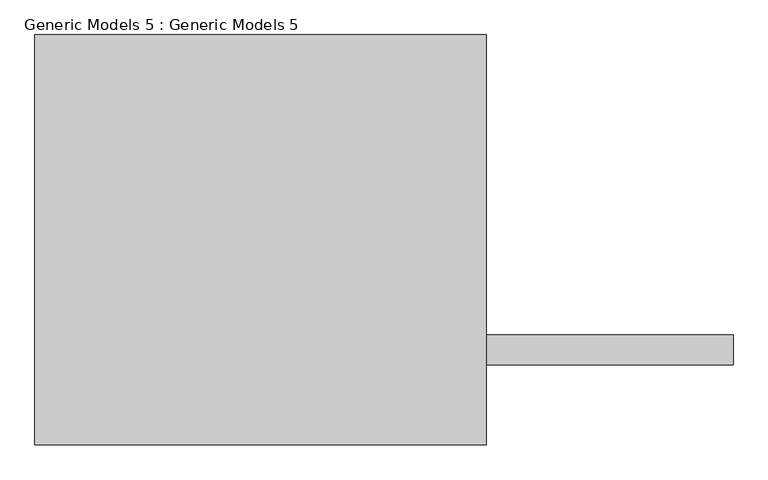
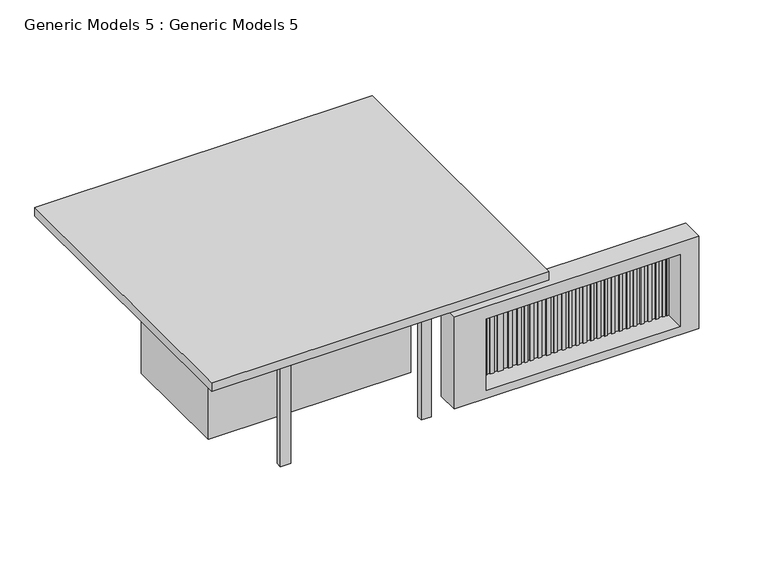
"""IFC4 building model written with IfcOpenShell, lengths in millimetres: proxy geometry, Generic Models 5 : Generic Models 5."""

from ifc_helpers import new_model, si_unit, frame, origin, place, context, project, spatial, polyline, outline, extrude, faceted_brep, source, transform, mapped, element, save


def generic_models_5_generic_models_5_ad9e1d00(model_context):
    return source(origin(), model_context, "Body", "SolidModel", [
        extrude(outline(polyline([(-17006.9161422, -10446.5171312), (-17006.9161422, -15983.7171312), (-23102.9161422, -15983.7171312), (-23102.9161422, -10446.5171312), (-17006.9161422, -10446.5171312)])), frame((0.0, 0.0, 9144.0), z_axis=(0.0, 0.0, 1.0), x_axis=(1.0, 0.0, 0.0)), (0.0, 0.0, 1.0), 166.4099226),
        extrude(outline(polyline([(-18692.6987295, -14904.2171312), (-18692.6987295, -14802.6171312), (-18514.8987295, -14802.6171312), (-18514.8987295, -14904.2171312), (-18692.6987295, -14904.2171312)])), frame((0.0, 0.0, 6400.8), z_axis=(0.0, 0.0, 1.0), x_axis=(1.0, 0.0, 0.0)), (0.0, 0.0, 1.0), 2743.2),
        extrude(outline(polyline([(-21238.3452638, -14904.2171312), (-21238.3452638, -14802.6171312), (-21055.1039169, -14802.6171312), (-21055.1039169, -14904.2171312), (-21238.3452638, -14904.2171312)])), frame((0.0, 0.0, 6400.8), z_axis=(0.0, 0.0, 1.0), x_axis=(1.0, 0.0, 0.0)), (0.0, 0.0, 1.0), 2743.2),
        extrude(outline(polyline([(-18188.0161422, -13700.4284904), (-21845.6161422, -13700.4284904), (-21845.6161422, -11605.6020297), (-18188.0161422, -11605.6020297), (-18188.0161422, -13700.4284904)])), frame((0.0, 0.0, 6400.8), z_axis=(0.0, 0.0, 1.0), x_axis=(1.0, 0.0, 0.0)), (0.0, 0.0, 1.0), 2743.2),
        faceted_brep([(-18092.8233, -14904.2171312, 8166.774585), (-13677.1878589, -14904.2171312, 8166.774585), (-13677.1878589, -14497.8171312, 8166.774585), (-18092.8233, -14497.8171312, 8166.774585), (-18092.8233, -14904.2171312, 6400.8), (-18092.8233, -14497.8171312, 6400.8), (-13677.1878589, -14497.8171312, 6400.8), (-13677.1878589, -14904.2171312, 6400.8), (-14010.7724772, -14904.2171312, 7924.7749037), (-14010.7724772, -14904.2171312, 6553.1749037), (-17515.9724772, -14904.2171312, 6553.1749037), (-17515.9724772, -14904.2171312, 7924.7749037), (-14010.7724772, -14548.6171312, 6553.1749037), (-14010.7724772, -14548.6171312, 7924.7749037), (-14050.845749, -14548.6171312, 7924.7749037), (-14050.845749, -14548.6171312, 6553.1749037), (-17304.418719, -14548.6171312, 7924.7749037), (-17439.1575133, -14548.6171312, 7924.7749037), (-17439.1575133, -14548.6171312, 6553.1749037), (-17304.418719, -14548.6171312, 6553.1749037), (-17164.8962989, -14548.6171312, 7924.7749037), (-17235.5161422, -14548.6171312, 7924.7749037), (-17235.5161422, -14548.6171312, 6553.1749037), (-17164.8962989, -14548.6171312, 6553.1749037), (-17006.9161422, -14548.6171312, 7924.7749037), (-17100.1180325, -14548.6171312, 7924.7749037), (-17100.1180325, -14548.6171312, 6553.1749037), (-17006.9161422, -14548.6171312, 6553.1749037), (-16841.0049665, -14548.6171312, 7924.7749037), (-16915.7491202, -14548.6171312, 7924.7749037), (-16915.7491202, -14548.6171312, 6553.1749037), (-16841.0049665, -14548.6171312, 6553.1749037), (-16681.5507721, -14548.6171312, 7924.7749037), (-16751.3119822, -14548.6171312, 7924.7749037), (-16751.3119822, -14548.6171312, 6553.1749037), (-16681.5507721, -14548.6171312, 6553.1749037), (-16561.3101772, -14548.6171312, 7924.7749037), (-16611.7895621, -14548.6171312, 7924.7749037), (-16611.7895621, -14548.6171312, 6553.1749037), (-16561.3101772, -14548.6171312, 6553.1749037), (-16452.9853168, -14548.6171312, 7924.7749037), (-16511.6161422, -14548.6171312, 7924.7749037), (-16511.6161422, -14548.6171312, 6553.1749037), (-16452.9853168, -14548.6171312, 6553.1749037), (-16305.6635068, -14548.6171312, 7924.7749037), (-16370.658423, -14548.6171312, 7924.7749037), (-16370.658423, -14548.6171312, 6553.1749037), (-16305.6635068, -14548.6171312, 6553.1749037), (-16149.6757079, -14548.6171312, 7924.7749037), (-16227.6696074, -14548.6171312, 7924.7749037), (-16227.6696074, -14548.6171312, 6553.1749037), (-16149.6757079, -14548.6171312, 6553.1749037), (-16024.0188699, -14548.6171312, 7924.7749037), (-16080.3477973, -14548.6171312, 7924.7749037), (-16080.3477973, -14548.6171312, 6553.1749037), (-16024.0188699, -14548.6171312, 6553.1749037), (-15872.3640655, -14548.6171312, 7924.7749037), (-15937.3589817, -14548.6171312, 7924.7749037), (-15937.3589817, -14548.6171312, 6553.1749037), (-15872.3640655, -14548.6171312, 6553.1749037), (-15763.3724772, -14548.6171312, 7924.7749037), (-15807.3691493, -14548.6171312, 7924.7749037), (-15807.3691493, -14548.6171312, 6553.1749037), (-15763.3724772, -14548.6171312, 6553.1749037), (-15631.207125, -14548.6171312, 7924.7749037), (-15683.203058, -14548.6171312, 7924.7749037), (-15683.203058, -14548.6171312, 6553.1749037), (-15631.207125, -14548.6171312, 6553.1749037), (-15496.8842982, -14548.6171312, 7924.7749037), (-15553.2132256, -14548.6171312, 7924.7749037), (-15553.2132256, -14548.6171312, 6553.1749037), (-15496.8842982, -14548.6171312, 6553.1749037), (-15371.2274602, -14548.6171312, 7924.7749037), (-15423.2233932, -14548.6171312, 7924.7749037), (-15423.2233932, -14548.6171312, 6553.1749037), (-15371.2274602, -14548.6171312, 6553.1749037), (-15241.2376278, -14548.6171312, 7924.7749037), (-15301.8995496, -14548.6171312, 7924.7749037), (-15301.8995496, -14548.6171312, 6553.1749037), (-15241.2376278, -14548.6171312, 6553.1749037), (-15119.9137842, -14548.6171312, 7924.7749037), (-15171.9097172, -14548.6171312, 7924.7749037), (-15171.9097172, -14548.6171312, 6553.1749037), (-15119.9137842, -14548.6171312, 6553.1749037), (-14985.5909574, -14548.6171312, 7924.7749037), (-15041.9198848, -14548.6171312, 7924.7749037), (-15041.9198848, -14548.6171312, 6553.1749037), (-14985.5909574, -14548.6171312, 6553.1749037), (-14851.2681306, -14548.6171312, 7924.7749037), (-14907.597058, -14548.6171312, 7924.7749037), (-14907.597058, -14548.6171312, 6553.1749037), (-14851.2681306, -14548.6171312, 6553.1749037), (-14712.6123094, -14548.6171312, 7924.7749037), (-14773.2742312, -14548.6171312, 7924.7749037), (-14773.2742312, -14548.6171312, 6553.1749037), (-14712.6123094, -14548.6171312, 6553.1749037), (-14591.2884658, -14548.6171312, 7924.7749037), (-14643.2843988, -14548.6171312, 7924.7749037), (-14643.2843988, -14548.6171312, 6553.1749037), (-14591.2884658, -14548.6171312, 6553.1749037), (-14459.1847676, -14548.6171312, 7924.7749037), (-14521.9605552, -14548.6171312, 7924.7749037), (-14521.9605552, -14548.6171312, 6553.1749037), (-14459.1847676, -14548.6171312, 6553.1749037), (-14322.6428122, -14548.6171312, 7924.7749037), (-14378.0161422, -14548.6171312, 7924.7749037), (-14378.0161422, -14548.6171312, 6553.1749037), (-14322.6428122, -14548.6171312, 6553.1749037), (-14196.9859742, -14548.6171312, 7924.7749037), (-14248.9819072, -14548.6171312, 7924.7749037), (-14248.9819072, -14548.6171312, 6553.1749037), (-14196.9859742, -14548.6171312, 6553.1749037), (-14074.454319, -14548.6171312, 7924.7749037), (-14118.9920748, -14548.6171312, 7924.7749037), (-14118.9920748, -14548.6171312, 6553.1749037), (-14074.454319, -14548.6171312, 6553.1749037), (-14050.845749, -14523.2171312, 6553.1749037), (-14074.454319, -14523.2171312, 6553.1749037), (-14118.9920748, -14523.2171312, 6553.1749037), (-14196.9859742, -14523.2171312, 6553.1749037), (-14248.9819072, -14523.2171312, 6553.1749037), (-14322.6428122, -14523.2171312, 6553.1749037), (-14378.0161422, -14523.2171312, 6553.1749037), (-14459.1847676, -14523.2171312, 6553.1749037), (-14521.9605552, -14523.2171312, 6553.1749037), (-14591.2884658, -14523.2171312, 6553.1749037), (-14643.2843988, -14523.2171312, 6553.1749037), (-14712.6123094, -14523.2171312, 6553.1749037), (-14773.2742312, -14523.2171312, 6553.1749037), (-14851.2681306, -14523.2171312, 6553.1749037), (-14907.597058, -14523.2171312, 6553.1749037), (-14985.5909574, -14523.2171312, 6553.1749037), (-15041.9198848, -14523.2171312, 6553.1749037), (-15119.9137842, -14523.2171312, 6553.1749037), (-15171.9097172, -14523.2171312, 6553.1749037), (-15241.2376278, -14523.2171312, 6553.1749037), (-15301.8995496, -14523.2171312, 6553.1749037), (-15371.2274602, -14523.2171312, 6553.1749037), (-15423.2233932, -14523.2171312, 6553.1749037), (-15496.8842982, -14523.2171312, 6553.1749037), (-15553.2132256, -14523.2171312, 6553.1749037), (-15631.207125, -14523.2171312, 6553.1749037), (-15683.203058, -14523.2171312, 6553.1749037), (-15763.3724772, -14523.2171312, 6553.1749037), (-15807.3691493, -14523.2171312, 6553.1749037), (-15872.3640655, -14523.2171312, 6553.1749037), (-15937.3589817, -14523.2171312, 6553.1749037), (-16024.0188699, -14523.2171312, 6553.1749037), (-16080.3477973, -14523.2171312, 6553.1749037), (-16149.6757079, -14523.2171312, 6553.1749037), (-16227.6696074, -14523.2171312, 6553.1749037), (-16305.6635068, -14523.2171312, 6553.1749037), (-16370.658423, -14523.2171312, 6553.1749037), (-16452.9853168, -14523.2171312, 6553.1749037), (-16511.6161422, -14523.2171312, 6553.1749037), (-16561.3101772, -14523.2171312, 6553.1749037), (-16611.7895621, -14523.2171312, 6553.1749037), (-16681.5507721, -14523.2171312, 6553.1749037), (-16751.3119822, -14523.2171312, 6553.1749037), (-16841.0049665, -14523.2171312, 6553.1749037), (-16915.7491202, -14523.2171312, 6553.1749037), (-17006.9161422, -14523.2171312, 6553.1749037), (-17100.1180325, -14523.2171312, 6553.1749037), (-17164.8962989, -14523.2171312, 6553.1749037), (-17235.5161422, -14523.2171312, 6553.1749037), (-17304.418719, -14523.2171312, 6553.1749037), (-17439.1575133, -14523.2171312, 6553.1749037), (-17633.6484681, -14523.2171312, 6553.1749037), (-17633.6484681, -14548.6171312, 6553.1749037), (-17515.9724772, -14548.6171312, 6553.1749037), (-17515.9724772, -14548.6171312, 7924.7749037), (-17633.6484681, -14548.6171312, 7924.7749037), (-17633.6484681, -14523.2171312, 7924.7749037), (-17439.1575133, -14523.2171312, 7924.7749037), (-17304.418719, -14523.2171312, 7924.7749037), (-17235.5161422, -14523.2171312, 7924.7749037), (-17164.8962989, -14523.2171312, 7924.7749037), (-17100.1180325, -14523.2171312, 7924.7749037), (-17006.9161422, -14523.2171312, 7924.7749037), (-16915.7491202, -14523.2171312, 7924.7749037), (-16841.0049665, -14523.2171312, 7924.7749037), (-16751.3119822, -14523.2171312, 7924.7749037), (-16681.5507721, -14523.2171312, 7924.7749037), (-16611.7895621, -14523.2171312, 7924.7749037), (-16561.3101772, -14523.2171312, 7924.7749037), (-16511.6161422, -14523.2171312, 7924.7749037), (-16452.9853168, -14523.2171312, 7924.7749037), (-16370.658423, -14523.2171312, 7924.7749037), (-16305.6635068, -14523.2171312, 7924.7749037), (-16227.6696074, -14523.2171312, 7924.7749037), (-16149.6757079, -14523.2171312, 7924.7749037), (-16080.3477973, -14523.2171312, 7924.7749037), (-16024.0188699, -14523.2171312, 7924.7749037), (-15937.3589817, -14523.2171312, 7924.7749037), (-15872.3640655, -14523.2171312, 7924.7749037), (-15807.3691493, -14523.2171312, 7924.7749037), (-15763.3724772, -14523.2171312, 7924.7749037), (-15683.203058, -14523.2171312, 7924.7749037), (-15631.207125, -14523.2171312, 7924.7749037), (-15553.2132256, -14523.2171312, 7924.7749037), (-15496.8842982, -14523.2171312, 7924.7749037), (-15423.2233932, -14523.2171312, 7924.7749037), (-15371.2274602, -14523.2171312, 7924.7749037), (-15301.8995496, -14523.2171312, 7924.7749037), (-15241.2376278, -14523.2171312, 7924.7749037), (-15171.9097172, -14523.2171312, 7924.7749037), (-15119.9137842, -14523.2171312, 7924.7749037), (-15041.9198848, -14523.2171312, 7924.7749037), (-14985.5909574, -14523.2171312, 7924.7749037), (-14907.597058, -14523.2171312, 7924.7749037), (-14851.2681306, -14523.2171312, 7924.7749037), (-14773.2742312, -14523.2171312, 7924.7749037), (-14712.6123094, -14523.2171312, 7924.7749037), (-14643.2843988, -14523.2171312, 7924.7749037), (-14591.2884658, -14523.2171312, 7924.7749037), (-14521.9605552, -14523.2171312, 7924.7749037), (-14459.1847676, -14523.2171312, 7924.7749037), (-14378.0161422, -14523.2171312, 7924.7749037), (-14322.6428122, -14523.2171312, 7924.7749037), (-14248.9819072, -14523.2171312, 7924.7749037), (-14196.9859742, -14523.2171312, 7924.7749037), (-14118.9920748, -14523.2171312, 7924.7749037), (-14074.454319, -14523.2171312, 7924.7749037), (-14050.845749, -14523.2171312, 7924.7749037)], [[[0, 1, 2, 3]], [[4, 5, 6, 7]], [[1, 0, 4, 7], [8, 9, 10, 11]], [[2, 1, 7, 6]], [[3, 2, 6, 5]], [[0, 3, 5, 4]], [[12, 13, 14, 15]], [[16, 17, 18, 19]], [[20, 21, 22, 23]], [[24, 25, 26, 27]], [[28, 29, 30, 31]], [[32, 33, 34, 35]], [[36, 37, 38, 39]], [[40, 41, 42, 43]], [[44, 45, 46, 47]], [[48, 49, 50, 51]], [[52, 53, 54, 55]], [[56, 57, 58, 59]], [[60, 61, 62, 63]], [[64, 65, 66, 67]], [[68, 69, 70, 71]], [[72, 73, 74, 75]], [[76, 77, 78, 79]], [[80, 81, 82, 83]], [[84, 85, 86, 87]], [[88, 89, 90, 91]], [[92, 93, 94, 95]], [[96, 97, 98, 99]], [[100, 101, 102, 103]], [[104, 105, 106, 107]], [[108, 109, 110, 111]], [[112, 113, 114, 115]], [[13, 12, 9, 8]], [[9, 12, 15, 116, 117, 115, 114, 118, 119, 111, 110, 120, 121, 107, 106, 122, 123, 103, 102, 124, 125, 99, 98, 126, 127, 95, 94, 128, 129, 91, 90, 130, 131, 87, 86, 132, 133, 83, 82, 134, 135, 79, 78, 136, 137, 75, 74, 138, 139, 71, 70, 140, 141, 67, 66, 142, 143, 63, 62, 144, 145, 59, 58, 146, 147, 55, 54, 148, 149, 51, 50, 150, 151, 47, 46, 152, 153, 43, 42, 154, 155, 39, 38, 156, 157, 35, 34, 158, 159, 31, 30, 160, 161, 27, 26, 162, 163, 23, 22, 164, 165, 19, 18, 166, 167, 168, 169, 10]], [[10, 169, 170, 11]], [[13, 8, 11, 170, 171, 172, 173, 17, 16, 174, 175, 21, 20, 176, 177, 25, 24, 178, 179, 29, 28, 180, 181, 33, 32, 182, 183, 37, 36, 184, 185, 41, 40, 186, 187, 45, 44, 188, 189, 49, 48, 190, 191, 53, 52, 192, 193, 57, 56, 194, 195, 61, 60, 196, 197, 65, 64, 198, 199, 69, 68, 200, 201, 73, 72, 202, 203, 77, 76, 204, 205, 81, 80, 206, 207, 85, 84, 208, 209, 89, 88, 210, 211, 93, 92, 212, 213, 97, 96, 214, 215, 101, 100, 216, 217, 105, 104, 218, 219, 109, 108, 220, 221, 113, 112, 222, 223, 14]], [[175, 174, 165, 164]], [[177, 176, 163, 162]], [[179, 178, 161, 160]], [[181, 180, 159, 158]], [[183, 182, 157, 156]], [[185, 184, 155, 154]], [[187, 186, 153, 152]], [[189, 188, 151, 150]], [[191, 190, 149, 148]], [[193, 192, 147, 146]], [[195, 194, 145, 144]], [[197, 196, 143, 142]], [[199, 198, 141, 140]], [[201, 200, 139, 138]], [[203, 202, 137, 136]], [[205, 204, 135, 134]], [[207, 206, 133, 132]], [[209, 208, 131, 130]], [[211, 210, 129, 128]], [[213, 212, 127, 126]], [[215, 214, 125, 124]], [[217, 216, 123, 122]], [[219, 218, 121, 120]], [[221, 220, 119, 118]], [[223, 222, 117, 116]], [[172, 167, 166, 173]], [[167, 172, 171, 168]], [[173, 166, 18, 17]], [[175, 164, 22, 21]], [[165, 174, 16, 19]], [[177, 162, 26, 25]], [[163, 176, 20, 23]], [[179, 160, 30, 29]], [[161, 178, 24, 27]], [[181, 158, 34, 33]], [[159, 180, 28, 31]], [[183, 156, 38, 37]], [[157, 182, 32, 35]], [[185, 154, 42, 41]], [[155, 184, 36, 39]], [[187, 152, 46, 45]], [[153, 186, 40, 43]], [[189, 150, 50, 49]], [[151, 188, 44, 47]], [[191, 148, 54, 53]], [[149, 190, 48, 51]], [[193, 146, 58, 57]], [[147, 192, 52, 55]], [[195, 144, 62, 61]], [[145, 194, 56, 59]], [[197, 142, 66, 65]], [[143, 196, 60, 63]], [[199, 140, 70, 69]], [[141, 198, 64, 67]], [[201, 138, 74, 73]], [[139, 200, 68, 71]], [[203, 136, 78, 77]], [[137, 202, 72, 75]], [[205, 134, 82, 81]], [[135, 204, 76, 79]], [[207, 132, 86, 85]], [[133, 206, 80, 83]], [[209, 130, 90, 89]], [[131, 208, 84, 87]], [[211, 128, 94, 93]], [[129, 210, 88, 91]], [[213, 126, 98, 97]], [[127, 212, 92, 95]], [[215, 124, 102, 101]], [[125, 214, 96, 99]], [[217, 122, 106, 105]], [[123, 216, 100, 103]], [[219, 120, 110, 109]], [[121, 218, 104, 107]], [[221, 118, 114, 113]], [[119, 220, 108, 111]], [[223, 116, 15, 14]], [[117, 222, 112, 115]], [[168, 171, 170, 169]]]),
    ])


if __name__ == "__main__":
    model = new_model("IFC4")
    model_context = context("Model", 3, world=origin())
    ifc_project = project(units=[si_unit("LENGTHUNIT", "METRE", prefix="MILLI")], contexts=[model_context])
    site = spatial("IfcSite", under=ifc_project)
    building = spatial("IfcBuilding", under=site)
    placement = place(None, origin())
    generic_models_5_generic_models_5_shape = generic_models_5_generic_models_5_ad9e1d00(model_context)
    element("IfcBuildingElementProxy", 1, Name="Generic Models 5 : Generic Models 5", ObjectType="Generic Models 5 : Generic Models 5", at=placement, inside=building, context=model_context, shape_type="MappedRepresentation", body=[
        mapped(generic_models_5_generic_models_5_shape, transform((0.0, 0.0, 0.0), x_axis=(1.0, 0.0, 0.0), y_axis=(0.0, 1.0, 0.0), z_axis=(0.0, 0.0, 1.0))),
    ])
    save(model, "model.ifc")
